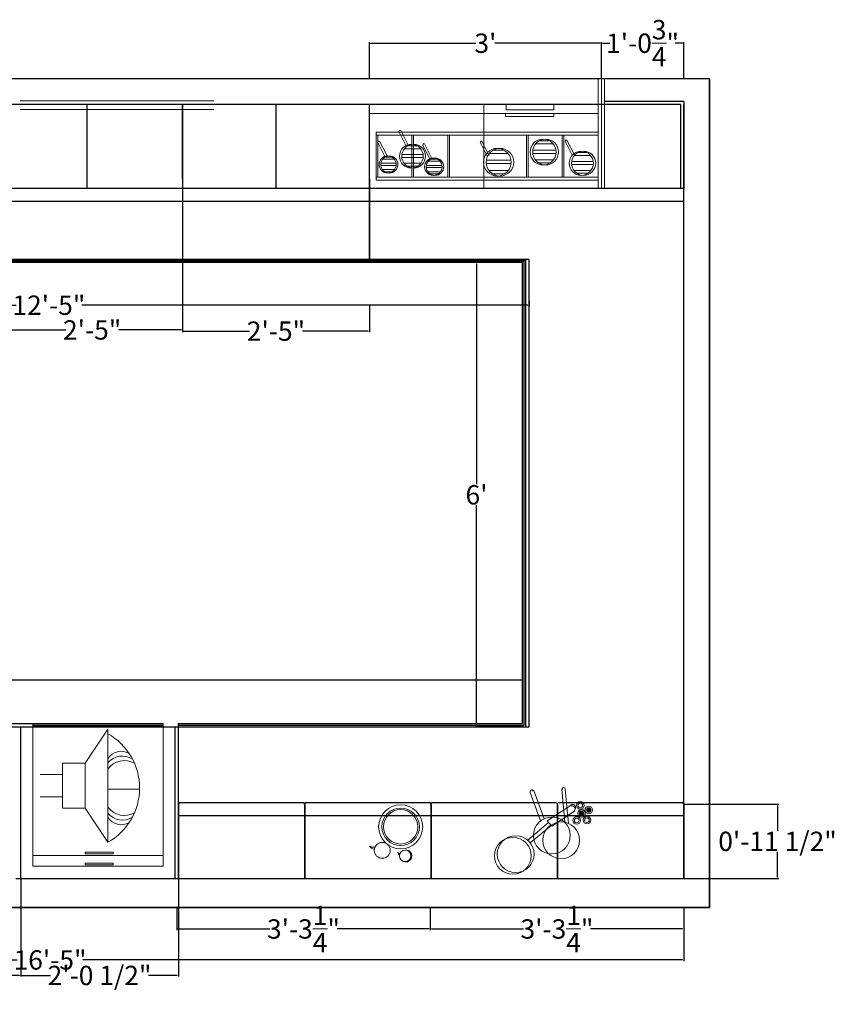
# Model space of a CAD drawing. Units: inches. Extents: x 1686244 to 1686928, y 1936095 to 1936489.
# Tile 11 of 11: x 1686801 to 1686928, y 1936330 to 1936483. Entities that reach past the tile are written whole.
import ezdxf

# ---------------------------------------------------------------- set-up
doc = ezdxf.new("R2010")
doc.units = ezdxf.units.IN
doc.header["$MEASUREMENT"] = 0
for name, color, linetype, lineweight in [('A-ANNO-DIMS', 240, 'Continuous', 18), ('A-CASE', 7, 'Continuous', 35), ('A-ELEV', 7, 'Continuous', 25), ('A-ELEV-PATT', 72, 'Continuous', 13), ('A-FURN', 40, 'Continuous', 18)]:
    doc.layers.add(name, color=color, linetype=linetype, lineweight=lineweight)
doc.styles.get("Standard").update_dxf_attribs({"font": 'arial.ttf'})
doc.dimstyles.get("Standard").update_dxf_attribs({"dimtxt": 3, "dimasz": 0.18, "dimexe": 0.18, "dimexo": 0.0625, "dimgap": 0.09, "dimtad": 0, "dimtih": 1, "dimtoh": 1, "dimzin": 0, "dimdsep": 46, "dimlunit": 4, "dimtxsty": 'Standard', "dimcen": 0.09, "dimadec": 0, "dimazin": 0, "dimtfac": 1, "dimtofl": 0, "dimtmove": 0, "dimatfit": 3, "dimfxl": 1, "dimtolj": 1, "dimtzin": 0, "dimarcsym": 0})

# ---------------------------------------------------------------- blocks, each defined once
blk = doc.blocks.new('*D21')
at = {"layer": 'A-ANNO-DIMS', "color": 0, "lineweight": -2, "transparency": 16777216}
for p, q in [((1686707.33, 1936344.88), (1686707.33, 1936336.62)), ((1686904.33, 1936344.88), (1686904.33, 1936336.62)), ((1686707.51, 1936336.8), (1686800.91, 1936336.8)), ((1686904.15, 1936336.8), (1686811.11, 1936336.8))]:
    blk.add_line(p, q, dxfattribs=at)
at = {"layer": 'A-ANNO-DIMS', "color": 0, "transparency": 16777216}
for points in [[(1686707.51, 1936336.83), (1686707.51, 1936336.77), (1686707.33, 1936336.8)], [(1686904.15, 1936336.83), (1686904.15, 1936336.77), (1686904.33, 1936336.8)]]:
    blk.add_solid(points, dxfattribs=at)
at = {"layer": 'Defpoints', "color": 0, "transparency": 16777216}
for p in [(1686707.33, 1936344.94), (1686904.33, 1936344.94), (1686904.33, 1936336.8)]:
    blk.add_point(p, dxfattribs=at)
at = {"layer": 'A-ANNO-DIMS', "color": 0, "transparency": 16777216, "insert": (1686806.01, 1936336.8), "char_height": 3, "attachment_point": 5}
blk.add_mtext('\\A1;16\'-5"', dxfattribs=at)
blk = doc.blocks.new('*D22')
at = {"layer": 'A-ANNO-DIMS', "color": 0, "lineweight": -2, "transparency": 16777216}
for p, q in [((1686865, 1936344.88), (1686865, 1936341.42)), ((1686904.33, 1936344.88), (1686904.33, 1936341.42)), ((1686865.18, 1936341.6), (1686879.45, 1936341.6)), ((1686904.15, 1936341.6), (1686889.88, 1936341.6))]:
    blk.add_line(p, q, dxfattribs=at)
at = {"layer": 'A-ANNO-DIMS', "color": 0, "transparency": 16777216}
for points in [[(1686865.18, 1936341.63), (1686865.18, 1936341.57), (1686865, 1936341.6)], [(1686904.15, 1936341.63), (1686904.15, 1936341.57), (1686904.33, 1936341.6)]]:
    blk.add_solid(points, dxfattribs=at)
at = {"layer": 'Defpoints', "color": 0, "transparency": 16777216}
for p in [(1686865, 1936344.94), (1686904.33, 1936344.94), (1686865, 1936341.6)]:
    blk.add_point(p, dxfattribs=at)
at = {"layer": 'A-ANNO-DIMS', "color": 0, "transparency": 16777216, "insert": (1686884.66, 1936341.6), "char_height": 3, "attachment_point": 5}
blk.add_mtext('\\A1;3\'-3{\\H1x;\\S1/4;}"', dxfattribs=at)
blk = doc.blocks.new('*D23')
at = {"layer": 'A-ANNO-DIMS', "color": 0, "lineweight": -2, "transparency": 16777216}
for p, q in [((1686825.67, 1936344.88), (1686825.67, 1936341.42)), ((1686865, 1936344.88), (1686865, 1936341.42)), ((1686825.85, 1936341.6), (1686840.12, 1936341.6)), ((1686864.82, 1936341.6), (1686850.55, 1936341.6))]:
    blk.add_line(p, q, dxfattribs=at)
at = {"layer": 'A-ANNO-DIMS', "color": 0, "transparency": 16777216}
for points in [[(1686825.85, 1936341.63), (1686825.85, 1936341.57), (1686825.67, 1936341.6)], [(1686864.82, 1936341.63), (1686864.82, 1936341.57), (1686865, 1936341.6)]]:
    blk.add_solid(points, dxfattribs=at)
at = {"layer": 'Defpoints', "color": 0, "transparency": 16777216}
for p in [(1686825.67, 1936344.94), (1686865, 1936344.94), (1686825.67, 1936341.6)]:
    blk.add_point(p, dxfattribs=at)
at = {"layer": 'A-ANNO-DIMS', "color": 0, "transparency": 16777216, "insert": (1686845.33, 1936341.6), "char_height": 3, "attachment_point": 5}
blk.add_mtext('\\A1;3\'-3{\\H1x;\\S1/4;}"', dxfattribs=at)
blk = doc.blocks.new('*D25')
at = {"layer": 'A-ANNO-DIMS', "color": 0, "lineweight": -2, "transparency": 16777216}
for p, q in [((1686879.26, 1936444.94), (1686872, 1936444.94)), ((1686872.18, 1936444.76), (1686872.18, 1936410.56)), ((1686872.18, 1936373.12), (1686872.18, 1936407.32)), ((1686879.4, 1936372.94), (1686872, 1936372.94))]:
    blk.add_line(p, q, dxfattribs=at)
at = {"layer": 'A-ANNO-DIMS', "color": 0, "transparency": 16777216}
for points in [[(1686872.15, 1936444.76), (1686872.21, 1936444.76), (1686872.18, 1936444.94)], [(1686872.15, 1936373.12), (1686872.21, 1936373.12), (1686872.18, 1936372.94)]]:
    blk.add_solid(points, dxfattribs=at)
at = {"layer": 'Defpoints', "color": 0, "transparency": 16777216}
for p in [(1686872.18, 1936444.94), (1686879.33, 1936444.94), (1686879.46, 1936372.94)]:
    blk.add_point(p, dxfattribs=at)
at = {"layer": 'A-ANNO-DIMS', "color": 0, "transparency": 16777216, "insert": (1686872.18, 1936408.94), "char_height": 3, "attachment_point": 5}
blk.add_mtext("\\A1;6'", dxfattribs=at)
blk = doc.blocks.new('*D26')
at = {"layer": 'A-ANNO-DIMS', "color": 0, "lineweight": -2, "transparency": 16777216}
for p, q in [((1686731.33, 1936439.01), (1686731.33, 1936438.16)), ((1686731.51, 1936438.34), (1686800.73, 1936438.34)), ((1686880.15, 1936438.34), (1686810.93, 1936438.34)), ((1686880.33, 1936439.01), (1686880.33, 1936438.16))]:
    blk.add_line(p, q, dxfattribs=at)
at = {"layer": 'A-ANNO-DIMS', "color": 0, "transparency": 16777216}
for points in [[(1686731.51, 1936438.37), (1686731.51, 1936438.31), (1686731.33, 1936438.34)], [(1686880.15, 1936438.37), (1686880.15, 1936438.31), (1686880.33, 1936438.34)]]:
    blk.add_solid(points, dxfattribs=at)
at = {"layer": 'Defpoints', "color": 0, "transparency": 16777216}
for p in [(1686731.33, 1936439.07), (1686731.33, 1936438.34), (1686880.33, 1936439.07)]:
    blk.add_point(p, dxfattribs=at)
at = {"layer": 'A-ANNO-DIMS', "color": 0, "transparency": 16777216, "insert": (1686805.83, 1936438.34), "char_height": 3, "attachment_point": 5}
blk.add_mtext('\\A1;12\'-5"', dxfattribs=at)
blk = doc.blocks.new('*D29')
at = {"layer": 'A-ANNO-DIMS', "color": 0, "lineweight": -2, "transparency": 16777216}
for p, q in [((1686797.56, 1936438.28), (1686797.56, 1936434.32)), ((1686826.56, 1936438.28), (1686826.56, 1936434.32)), ((1686797.74, 1936434.5), (1686808.44, 1936434.5)), ((1686826.38, 1936434.5), (1686816.65, 1936434.5))]:
    blk.add_line(p, q, dxfattribs=at)
at = {"layer": 'A-ANNO-DIMS', "color": 0, "transparency": 16777216}
for points in [[(1686797.74, 1936434.53), (1686797.74, 1936434.47), (1686797.56, 1936434.5)], [(1686826.38, 1936434.53), (1686826.38, 1936434.47), (1686826.56, 1936434.5)]]:
    blk.add_solid(points, dxfattribs=at)
at = {"layer": 'Defpoints', "color": 0, "transparency": 16777216}
for p in [(1686797.56, 1936438.34), (1686826.56, 1936438.34), (1686826.56, 1936434.5)]:
    blk.add_point(p, dxfattribs=at)
at = {"layer": 'A-ANNO-DIMS', "color": 0, "transparency": 16777216, "insert": (1686812.54, 1936434.5), "char_height": 3, "attachment_point": 5}
blk.add_mtext('\\A1;2\'-5"', dxfattribs=at)
blk = doc.blocks.new('*D30')
at = {"layer": 'A-ANNO-DIMS', "color": 0, "lineweight": -2, "transparency": 16777216}
for p, q in [((1686826.56, 1936438.28), (1686826.56, 1936434.14)), ((1686855.56, 1936438.28), (1686855.56, 1936434.14)), ((1686826.74, 1936434.32), (1686836.95, 1936434.32)), ((1686855.38, 1936434.32), (1686845.16, 1936434.32))]:
    blk.add_line(p, q, dxfattribs=at)
at = {"layer": 'A-ANNO-DIMS', "color": 0, "transparency": 16777216}
for points in [[(1686826.74, 1936434.35), (1686826.74, 1936434.29), (1686826.56, 1936434.32)], [(1686855.38, 1936434.35), (1686855.38, 1936434.29), (1686855.56, 1936434.32)]]:
    blk.add_solid(points, dxfattribs=at)
at = {"layer": 'Defpoints', "color": 0, "transparency": 16777216}
for p in [(1686826.56, 1936438.34), (1686855.56, 1936438.34), (1686855.56, 1936434.32)]:
    blk.add_point(p, dxfattribs=at)
at = {"layer": 'A-ANNO-DIMS', "color": 0, "transparency": 16777216, "insert": (1686841.06, 1936434.32), "char_height": 3, "attachment_point": 5}
blk.add_mtext('\\A1;2\'-5"', dxfattribs=at)
blk = doc.blocks.new('*D31')
at = {"layer": 'A-ANNO-DIMS', "color": 0, "lineweight": -2, "transparency": 16777216}
for p, q in [((1686855.56, 1936473.5), (1686855.56, 1936479.15)), ((1686891.56, 1936473.5), (1686891.56, 1936479.15)), ((1686855.74, 1936478.97), (1686872.09, 1936478.97)), ((1686891.38, 1936478.97), (1686875.03, 1936478.97))]:
    blk.add_line(p, q, dxfattribs=at)
at = {"layer": 'A-ANNO-DIMS', "color": 0, "transparency": 16777216}
for points in [[(1686855.74, 1936479), (1686855.74, 1936478.94), (1686855.56, 1936478.97)], [(1686891.38, 1936479), (1686891.38, 1936478.94), (1686891.56, 1936478.97)]]:
    blk.add_solid(points, dxfattribs=at)
at = {"layer": 'Defpoints', "color": 0, "transparency": 16777216}
for p in [(1686891.56, 1936478.97), (1686855.56, 1936473.44), (1686891.56, 1936473.44)]:
    blk.add_point(p, dxfattribs=at)
at = {"layer": 'A-ANNO-DIMS', "color": 0, "transparency": 16777216, "insert": (1686873.56, 1936478.97), "char_height": 3, "attachment_point": 5}
blk.add_mtext("\\A1;3'", dxfattribs=at)
blk = doc.blocks.new('*D32')
at = {"layer": 'A-ANNO-DIMS', "color": 0, "lineweight": -2, "transparency": 16777216}
for p, q in [((1686891.56, 1936473.5), (1686891.56, 1936479.15)), ((1686904.33, 1936473.5), (1686904.33, 1936479.15)), ((1686891.74, 1936478.97), (1686892.87, 1936478.97)), ((1686904.15, 1936478.97), (1686903.02, 1936478.97))]:
    blk.add_line(p, q, dxfattribs=at)
at = {"layer": 'A-ANNO-DIMS', "color": 0, "transparency": 16777216}
for points in [[(1686891.74, 1936479), (1686891.74, 1936478.94), (1686891.56, 1936478.97)], [(1686904.15, 1936479), (1686904.15, 1936478.94), (1686904.33, 1936478.97)]]:
    blk.add_solid(points, dxfattribs=at)
at = {"layer": 'Defpoints', "color": 0, "transparency": 16777216}
for p in [(1686904.33, 1936478.97), (1686891.56, 1936473.44), (1686904.33, 1936473.44)]:
    blk.add_point(p, dxfattribs=at)
at = {"layer": 'A-ANNO-DIMS', "color": 0, "transparency": 16777216, "insert": (1686897.94, 1936478.97), "char_height": 3, "attachment_point": 5}
blk.add_mtext('\\A1;1\'-0{\\H1x;\\S3/4;}"', dxfattribs=at)
blk = doc.blocks.new('*D35')
at = {"layer": 'A-ANNO-DIMS', "color": 0, "lineweight": -2, "transparency": 16777216}
for p, q in [((1686707.33, 1936377.76), (1686707.33, 1936380.38)), ((1686707.51, 1936380.2), (1686788.23, 1936380.2)), ((1686879.15, 1936380.2), (1686798.43, 1936380.2)), ((1686879.33, 1936377.76), (1686879.33, 1936380.38))]:
    blk.add_line(p, q, dxfattribs=at)
at = {"layer": 'A-ANNO-DIMS', "color": 0, "transparency": 16777216}
for points in [[(1686707.51, 1936380.23), (1686707.51, 1936380.17), (1686707.33, 1936380.2)], [(1686879.15, 1936380.23), (1686879.15, 1936380.17), (1686879.33, 1936380.2)]]:
    blk.add_solid(points, dxfattribs=at)
at = {"layer": 'Defpoints', "color": 0, "transparency": 16777216}
for p in [(1686879.33, 1936380.2), (1686707.33, 1936377.7), (1686879.33, 1936377.7)]:
    blk.add_point(p, dxfattribs=at)
at = {"layer": 'A-ANNO-DIMS', "color": 0, "transparency": 16777216, "insert": (1686793.33, 1936380.2), "char_height": 3, "attachment_point": 5}
blk.add_mtext('\\A1;14\'-4"', dxfattribs=at)
blk = doc.blocks.new('*D108')
at = {"layer": 'A-ANNO-DIMS', "color": 0, "lineweight": -2, "transparency": 16777216}
for p, q in [((1686776.77, 1936349.38), (1686776.77, 1936334.21)), ((1686801.47, 1936349.38), (1686801.47, 1936334.21)), ((1686776.95, 1936334.39), (1686781.52, 1936334.39)), ((1686801.29, 1936334.39), (1686796.72, 1936334.39))]:
    blk.add_line(p, q, dxfattribs=at)
at = {"layer": 'A-ANNO-DIMS', "color": 0, "transparency": 16777216}
for points in [[(1686776.95, 1936334.42), (1686776.95, 1936334.36), (1686776.77, 1936334.39)], [(1686801.29, 1936334.42), (1686801.29, 1936334.36), (1686801.47, 1936334.39)]]:
    blk.add_solid(points, dxfattribs=at)
at = {"layer": 'Defpoints', "color": 0, "transparency": 16777216}
for p in [(1686776.77, 1936349.44), (1686801.47, 1936349.44), (1686801.47, 1936334.39)]:
    blk.add_point(p, dxfattribs=at)
at = {"layer": 'A-ANNO-DIMS', "color": 0, "transparency": 16777216, "insert": (1686789.12, 1936334.39), "char_height": 3, "attachment_point": 5}
blk.add_mtext('\\A1;2\'-0 1/2"', dxfattribs=at)
blk = doc.blocks.new('*D109')
at = {"layer": 'A-ANNO-DIMS', "color": 0, "lineweight": -2, "transparency": 16777216}
for p, q in [((1686801.47, 1936349.38), (1686801.47, 1936334.21)), ((1686825.92, 1936349.38), (1686825.92, 1936334.21)), ((1686801.65, 1936334.39), (1686806.1, 1936334.39)), ((1686825.74, 1936334.39), (1686821.29, 1936334.39))]:
    blk.add_line(p, q, dxfattribs=at)
at = {"layer": 'A-ANNO-DIMS', "color": 0, "transparency": 16777216}
for points in [[(1686801.65, 1936334.42), (1686801.65, 1936334.36), (1686801.47, 1936334.39)], [(1686825.74, 1936334.42), (1686825.74, 1936334.36), (1686825.92, 1936334.39)]]:
    blk.add_solid(points, dxfattribs=at)
at = {"layer": 'Defpoints', "color": 0, "transparency": 16777216}
for p in [(1686801.47, 1936349.44), (1686825.92, 1936349.44), (1686825.92, 1936334.39)]:
    blk.add_point(p, dxfattribs=at)
at = {"layer": 'A-ANNO-DIMS', "color": 0, "transparency": 16777216, "insert": (1686813.69, 1936334.39), "char_height": 3, "attachment_point": 5}
blk.add_mtext('\\A1;2\'-0 1/2"', dxfattribs=at)
blk = doc.blocks.new('*D112')
at = {"layer": 'A-ANNO-DIMS', "color": 0, "lineweight": -2, "transparency": 16777216}
for p, q in [((1686904.39, 1936360.94), (1686919.06, 1936360.94)), ((1686918.88, 1936360.76), (1686918.88, 1936356.83)), ((1686918.88, 1936349.62), (1686918.88, 1936353.55)), ((1686904.39, 1936349.44), (1686919.06, 1936349.44))]:
    blk.add_line(p, q, dxfattribs=at)
at = {"layer": 'A-ANNO-DIMS', "color": 0, "transparency": 16777216}
for points in [[(1686918.85, 1936360.76), (1686918.91, 1936360.76), (1686918.88, 1936360.94)], [(1686918.85, 1936349.62), (1686918.91, 1936349.62), (1686918.88, 1936349.44)]]:
    blk.add_solid(points, dxfattribs=at)
at = {"layer": 'Defpoints', "color": 0, "transparency": 16777216}
for p in [(1686904.33, 1936360.94), (1686904.33, 1936349.44), (1686918.88, 1936349.44)]:
    blk.add_point(p, dxfattribs=at)
at = {"layer": 'A-ANNO-DIMS', "color": 0, "transparency": 16777216, "insert": (1686918.88, 1936355.19), "char_height": 3, "attachment_point": 5}
blk.add_mtext('\\A1;0\'-11 1/2"', dxfattribs=at)

msp = doc.modelspace()

# ---------------------------------------------------------------- hatches: boundary and pattern name
at = {"layer": 'A-ELEV-PATT'}
h = msp.add_hatch(dxfattribs=at)
h.set_pattern_fill('ANSI32', color=256, scale=3.918348, angle=135)
h.set_pattern_definition([(180, (-855412.5119, -981919.0557), (-2e-16, -1.46938062567), []), (180, (-855413.0017, -981918.5659), (-2e-16, -1.46938062567), [])])
h.paths.add_polyline_path([(1686882.705, 1936460.094, 0.3861806), (1686884.519, 1936462.092, 0.3861806), (1686882.705, 1936464.09, 0.3861806), (1686880.892, 1936462.092, 0.3861806)])
h = msp.add_hatch(dxfattribs=at)
h.set_pattern_fill('ANSI32', color=256, scale=3.601818, angle=135)
h.set_pattern_definition([(180, (-650062.0521, -746167.9158), (-2e-16, -1.3506815667), []), (180, (-650062.5023, -746167.4655), (-2e-16, -1.3506815667), [])])
h.paths.add_polyline_path([(1686862.246, 1936459.617, 0.3861806), (1686863.913, 1936461.453, 0.3861806), (1686862.246, 1936463.29, 0.3861806), (1686860.579, 1936461.453, 0.3861806)])
h = msp.add_hatch(dxfattribs=at)
h.set_pattern_fill('ANSI32', color=256, scale=4.184979, angle=135)
h.set_pattern_definition([(180, (-1028414.4015, -1180506.824), (-2e-16, -1.5693671227), []), (180, (-1028414.9246, -1180506.3008), (-2e-16, -1.5693671227), [])])
h.paths.add_polyline_path([(1686875.606, 1936458.385, 0.3861806), (1686877.543, 1936460.519, 0.3861806), (1686875.606, 1936462.653, 0.3861806), (1686873.669, 1936460.519, 0.3861806)])
h = msp.add_hatch(dxfattribs=at)
h.set_pattern_fill('ANSI32', color=256, scale=2.6, angle=135)
h.set_pattern_definition([(180, (-68.4762, -16.7264), (-1e-16, -0.975), []), (180, (-68.8012, -16.4014), (-1e-16, -0.975), [])])
h.paths.add_polyline_path([(1686858.514, 1936458.834, 0.3861806), (1686859.718, 1936460.16, 0.3861806), (1686858.514, 1936461.486, 0.3861806), (1686857.311, 1936460.16, 0.3861806)])
h = msp.add_hatch(dxfattribs=at)
h.set_pattern_fill('ANSI32', color=256, scale=2.637795, angle=135)
h.set_pattern_definition([(180, (-24583.2303, -28166.474), (-1e-16, -0.98917299), []), (180, (-24583.5601, -28166.1443), (-1e-16, -0.98917299), [])])
h.paths.add_polyline_path([(1686865.606, 1936458.47, 0.3861806), (1686866.827, 1936459.815, 0.3861806), (1686865.606, 1936461.16, 0.3861806), (1686864.385, 1936459.815, 0.3861806)])
h = msp.add_hatch(dxfattribs=at)
h.set_pattern_fill('ANSI32', color=256, scale=3.669954, angle=135)
h.set_pattern_definition([(180, (-694244.093, -796917.2364), (-2e-16, -1.3762328775), []), (180, (-694244.5517, -796916.7777), (-2e-16, -1.3762328775), [])])
h.paths.add_polyline_path([(1686888.611, 1936458.49, 0.3861806), (1686890.31, 1936460.361, 0.3861806), (1686888.611, 1936462.232, 0.3861806), (1686886.912, 1936460.361, 0.3861806)])

# ---------------------------------------------------------------- linework, layer by layer
at = {"layer": 'A-CASE'}
for p, q in [((1686908.327, 1936344.942), (1686908.327, 1936473.442)), ((1686703.327, 1936344.942), (1686908.327, 1936344.942))]:
    msp.add_line(p, q, dxfattribs=at)
at = {"layer": 'A-ELEV'}
for p, q in [((1686908.327, 1936473.442), (1686703.327, 1936473.442)), ((1686903.827, 1936469.442), (1686707.327, 1936469.442)), ((1686811.775, 1936456.442), (1686811.775, 1936469.442)), ((1686826.556, 1936457.879), (1686826.556, 1936469.442)), ((1686826.556, 1936469.442), (1686826.556, 1936438.341)), ((1686841.106, 1936456.442), (1686841.106, 1936469.442)), ((1686855.556, 1936444.942), (1686855.556, 1936469.442)), ((1686904.327, 1936469.942), (1686892.056, 1936469.942)), ((1686903.827, 1936469.442), (1686903.827, 1936456.442)), ((1686904.327, 1936469.942), (1686904.327, 1936456.442)), ((1686904.327, 1936349.442), (1686904.327, 1936469.442)), ((1686855.556, 1936457.909), (1686855.556, 1936444.942)), ((1686904.327, 1936456.442), (1686731.327, 1936456.442)), ((1686904.327, 1936454.442), (1686731.327, 1936454.442)), ((1686880.327, 1936445.442), (1686731.327, 1936445.442)), ((1686879.827, 1936445.342), (1686731.327, 1936445.342)), ((1686879.577, 1936445.097), (1686731.327, 1936445.097)), ((1686879.327, 1936444.942), (1686731.327, 1936444.942)), ((1686879.327, 1936373.442), (1686879.327, 1936444.942)), ((1686879.577, 1936373.192), (1686879.577, 1936445.342)), ((1686879.827, 1936372.942), (1686879.827, 1936445.342)), ((1686880.327, 1936372.942), (1686880.327, 1936445.442)), ((1686752.327, 1936373.442), (1686823.58, 1936373.442)), ((1686752.327, 1936372.942), (1686880.327, 1936372.942)), ((1686801.471, 1936349.442), (1686801.471, 1936372.942)), ((1686825.419, 1936349.442), (1686825.419, 1936372.942)), ((1686825.919, 1936349.442), (1686825.919, 1936373.442)), ((1686825.919, 1936373.442), (1686879.327, 1936373.442)), ((1686825.919, 1936373.192), (1686879.577, 1936373.192)), ((1686826.169, 1936361.192), (1686845.271, 1936361.192)), ((1686845.771, 1936361.192), (1686864.873, 1936361.192)), ((1686865.373, 1936361.192), (1686884.475, 1936361.192)), ((1686884.975, 1936361.192), (1686904.077, 1936361.192)), ((1686904.327, 1936360.942), (1686904.327, 1936349.442)), ((1686825.919, 1936359.192), (1686904.327, 1936359.192)), ((1686800.704, 1936349.442), (1686904.327, 1936349.442))]:
    msp.add_line(p, q, dxfattribs=at)
at = {"layer": 'A-ELEV', "const_width": 0.25}
for points in [[(1686825.919, 1936360.942), (1686825.919, 1936349.442)], [(1686845.521, 1936360.942), (1686845.521, 1936349.442)], [(1686865.123, 1936360.942), (1686865.123, 1936349.442)], [(1686884.725, 1936360.942), (1686884.725, 1936349.442)]]:
    msp.add_lwpolyline(points, dxfattribs=at)
at = {"layer": 'A-ELEV'}
for centre, start, end in [((1686826.169, 1936360.942), 90, 180), ((1686845.271, 1936360.942), 0, 90), ((1686845.771, 1936360.942), 90, 180), ((1686864.873, 1936360.942), 0, 90), ((1686865.373, 1936360.942), 90, 180), ((1686904.077, 1936360.942), 0, 90)]:
    msp.add_arc(centre, 0.25, start, end, dxfattribs=at)
at = {"layer": 'A-FURN'}
for p, q in [((1686891.056, 1936473.442), (1686891.056, 1936456.442)), ((1686891.556, 1936473.442), (1686891.556, 1936456.442)), ((1686892.056, 1936473.442), (1686892.056, 1936456.442)), ((1686801.392, 1936470.034), (1686831.445, 1936470.034)), ((1686801.392, 1936468.712), (1686831.445, 1936468.712)), ((1686873.306, 1936456.442), (1686873.306, 1936469.442)), ((1686855.556, 1936468.059), (1686891.056, 1936468.059)), ((1686861.564, 1936463.164), (1686860.415, 1936465.436)), ((1686857.097, 1936464.701), (1686856.597, 1936464.701)), ((1686856.597, 1936464.701), (1686873.306, 1936464.701)), ((1686856.847, 1936464.701), (1686856.847, 1936458.206)), ((1686861.227, 1936463.096), (1686860.183, 1936465.159)), ((1686862.167, 1936464.701), (1686862.167, 1936458.206)), ((1686862.417, 1936464.701), (1686862.417, 1936458.206)), ((1686867.736, 1936464.701), (1686867.736, 1936458.206)), ((1686867.986, 1936464.701), (1686867.986, 1936458.206)), ((1686879.917, 1936464.701), (1686879.917, 1936458.206)), ((1686880.167, 1936464.701), (1686880.167, 1936458.206)), ((1686885.486, 1936464.701), (1686885.486, 1936458.206)), ((1686885.736, 1936464.701), (1686885.736, 1936458.206)), ((1686887.365, 1936461.682), (1686886.216, 1936463.953)), ((1686857.955, 1936461.42), (1686856.912, 1936463.484)), ((1686858.293, 1936461.489), (1686857.144, 1936463.76)), ((1686864.914, 1936461.044), (1686863.871, 1936463.108)), ((1686865.252, 1936461.112), (1686864.103, 1936463.384)), ((1686873.827, 1936461.453), (1686872.783, 1936463.517)), ((1686874.164, 1936461.521), (1686873.015, 1936463.793)), ((1686887.027, 1936461.613), (1686885.984, 1936463.677)), ((1686857.097, 1936458.206), (1686856.597, 1936458.206)), ((1686811.474, 1936367.336), (1686814.986, 1936372.603)), ((1686814.986, 1936355.046), (1686814.986, 1936372.603)), ((1686811.474, 1936367.336), (1686807.963, 1936367.336)), ((1686807.963, 1936367.336), (1686807.963, 1936360.313)), ((1686811.474, 1936360.313), (1686811.474, 1936367.336)), ((1686807.963, 1936365.58), (1686804.452, 1936365.58)), ((1686814.986, 1936363.289), (1686819.897, 1936363.289)), ((1686882.659, 1936358.693), (1686881.051, 1936363.082)), ((1686885.86, 1936358.156), (1686885.43, 1936363.303)), ((1686885.947, 1936363.303), (1686886.446, 1936357.975)), ((1686804.452, 1936362.069), (1686807.963, 1936362.069)), ((1686882.115, 1936358.36), (1686880.506, 1936362.748)), ((1686807.963, 1936360.313), (1686811.474, 1936360.313)), ((1686814.986, 1936355.046), (1686811.474, 1936360.313)), ((1686883.142, 1936358.367), (1686886.712, 1936360.68)), ((1686889.513, 1936360.072), (1686889.251, 1936360.128)), ((1686889.513, 1936360.035), (1686889.251, 1936359.979)), ((1686889.528, 1936360.107), (1686889.312, 1936360.264)), ((1686889.556, 1936360.132), (1686889.422, 1936360.364)), ((1686889.592, 1936360.144), (1686889.564, 1936360.41)), ((1686889.63, 1936360.14), (1686889.712, 1936360.394)), ((1686889.662, 1936360.121), (1686889.841, 1936360.32)), ((1686889.685, 1936360.09), (1686889.929, 1936360.199)), ((1686889.685, 1936360.017), (1686889.929, 1936359.908)), ((1686889.692, 1936360.054), (1686889.96, 1936360.054)), ((1686883.841, 1936357.559), (1686887.386, 1936359.891)), ((1686888.384, 1936359.548), (1686888.123, 1936359.604)), ((1686888.384, 1936359.51), (1686888.123, 1936359.455)), ((1686888.4, 1936359.583), (1686888.183, 1936359.74)), ((1686888.4, 1936359.476), (1686888.183, 1936359.319)), ((1686888.428, 1936359.608), (1686888.294, 1936359.84)), ((1686888.428, 1936359.451), (1686888.294, 1936359.219)), ((1686888.464, 1936359.62), (1686888.436, 1936359.886)), ((1686888.464, 1936359.439), (1686888.436, 1936359.173)), ((1686888.501, 1936359.616), (1686888.584, 1936359.87)), ((1686888.501, 1936359.443), (1686888.584, 1936359.189)), ((1686888.534, 1936359.597), (1686888.713, 1936359.796)), ((1686888.534, 1936359.462), (1686888.713, 1936359.263)), ((1686888.556, 1936359.566), (1686888.8, 1936359.675)), ((1686888.556, 1936359.492), (1686888.8, 1936359.384)), ((1686888.564, 1936359.529), (1686888.831, 1936359.529)), ((1686889.528, 1936360), (1686889.312, 1936359.843)), ((1686889.556, 1936359.975), (1686889.422, 1936359.743)), ((1686889.592, 1936359.963), (1686889.564, 1936359.697)), ((1686889.63, 1936359.967), (1686889.712, 1936359.713)), ((1686889.662, 1936359.986), (1686889.841, 1936359.787)), ((1686880.122, 1936355.373), (1686883.357, 1936358.113)), ((1686880.507, 1936354.968), (1686883.756, 1936357.656)), ((1686883.357, 1936358.113), (1686883.142, 1936358.367)), ((1686883.841, 1936357.559), (1686883.357, 1936358.113)), ((1686803.322, 1936353.022), (1686823.58, 1936353.022))]:
    msp.add_line(p, q, dxfattribs=at)
for points in [[(1686876.785, 1936469.442), (1686884.183, 1936469.442), (1686884.183, 1936468.656), (1686876.785, 1936468.656)], [(1686876.694, 1936468.059), (1686884.183, 1936468.059), (1686884.183, 1936467.63), (1686876.694, 1936467.63)], [(1686856.597, 1936465.201), (1686891.056, 1936465.201), (1686891.056, 1936457.706), (1686856.597, 1936457.706)], [(1686803.322, 1936373.442), (1686823.58, 1936373.442), (1686823.58, 1936351.331), (1686803.322, 1936351.331)], [(1686811.453, 1936353.524), (1686815.803, 1936353.524), (1686815.803, 1936353.234), (1686811.453, 1936353.234)], [(1686811.453, 1936351.82), (1686815.803, 1936351.82), (1686815.803, 1936351.531), (1686811.453, 1936351.531)]]:
    msp.add_lwpolyline(points, close=True, dxfattribs=at)
for points in [[(1686857.097, 1936464.701), (1686891.056, 1936464.701)], [(1686891.056, 1936458.206), (1686857.097, 1936458.206)]]:
    msp.add_lwpolyline(points, dxfattribs=at)
at = {"layer": 'A-FURN', "const_width": 0.25}
msp.add_lwpolyline([(1686803.322, 1936373.179), (1686823.58, 1936373.179)], dxfattribs=at)
at = {"layer": 'A-FURN'}
for centre, radius in [((1686882.512, 1936462.092), 2.007), ((1686882.899, 1936462.092), 2.007), ((1686862.068, 1936461.453), 1.845), ((1686862.424, 1936461.453), 1.845), ((1686875.399, 1936460.519), 2.144), ((1686875.813, 1936460.519), 2.144), ((1686858.386, 1936460.16), 1.332), ((1686858.643, 1936460.16), 1.332), ((1686865.475, 1936459.815), 1.351), ((1686865.736, 1936459.815), 1.351), ((1686888.43, 1936460.361), 1.88), ((1686888.792, 1936460.361), 1.88), ((1686880.881, 1936363.063), 0.058), ((1686885.473, 1936363.33), 0.0404), ((1686860.41, 1936357.443), 3.415), ((1686860.41, 1936357.443), 2.915), ((1686860.41, 1936357.443), 2.665), ((1686888.288, 1936360.768), 0.587), ((1686888.473, 1936359.529), 0.587), ((1686888.288, 1936360.768), 0.358), ((1686889.602, 1936360.054), 0.587), ((1686889.602, 1936360.054), 0.358), ((1686889.602, 1936360.054), 0.0908), ((1686883.87, 1936356.104), 2.858), ((1686887.732, 1936358.437), 0.587), ((1686887.732, 1936358.437), 0.358), ((1686888.473, 1936359.529), 0.358), ((1686888.473, 1936359.529), 0.0908), ((1686889.315, 1936358.485), 0.587), ((1686889.315, 1936358.485), 0.358), ((1686885.317, 1936355.35), 2.858), ((1686877.821, 1936352.955), 2.858), ((1686878.253, 1936353.212), 2.858), ((1686857.552, 1936353.787), 1.23), ((1686861.118, 1936352.952), 0.893)]:
    msp.add_circle(centre, radius, dxfattribs=at)
for centre, radius, start, end in [((1686860.337, 1936465.265), 0.187, 65.40581, 214.5723), ((1686886.138, 1936463.783), 0.187, 65.40581, 214.5723), ((1686857.066, 1936463.59), 0.187, 65.40581, 214.5723), ((1686864.025, 1936463.214), 0.187, 65.40581, 214.5723), ((1686872.937, 1936463.623), 0.187, 65.40581, 214.5723), ((1686810.237, 1936363.46), 9.662, 299.43944, 60.56056), ((1686817.055, 1936366.727), 2.43, 60.09039, 148.36141), ((1686817.222, 1936365.502), 2.922, 57.7978, 139.95062), ((1686817.533, 1936364.596), 3.126, 59.86609, 144.59682), ((1686880.82, 1936362.848), 0.329, 45.31397, 197.64967), ((1686885.688, 1936363.303), 0.259, 0, 180), ((1686817.533, 1936362.324), 3.126, 215.40318, 300.13391), ((1686884.475, 1936360.942), 0.25, 0, 90), ((1686884.975, 1936360.942), 0.25, 90, 180), ((1686887.108, 1936360.456), 0.455, 320.72145, 150.51859), ((1686886.911, 1936360.168), 0.55, 329.69008, 111.24004), ((1686817.222, 1936361.418), 2.922, 220.04938, 302.2022), ((1686817.055, 1936360.194), 2.43, 211.63859, 299.90961), ((1686856.445, 1936355.023), 1.034, 213.44944, 264.20204), ((1686856.387, 1936356.1), 1.832, 243.95895, 271.05946), ((1686860.317, 1936353.469), 0.35, 178.70944, 257.58249), ((1686860.206, 1936353.553), 0.251, 197.81344, 293.15493), ((1686860.206, 1936353.553), 0.251, 0.0117442645317992, 0.0117443708500602), ((1686861.22, 1936352.919), 0.932, 228.35416, 96.31644)]:
    msp.add_arc(centre, radius, start, end, dxfattribs=at)
for p in [(1686862.167, 1936464.701), (1686867.736, 1936464.701)]:
    msp.add_point(p, dxfattribs=at)

# ---------------------------------------------------------------- dimensions: what is measured, and where the dimension line sits
at = {"layer": 'A-ANNO-DIMS'}
for base, p1, p2, override, picture, middle in [((1686904.327, 1936478.966), (1686891.556, 1936473.442), (1686904.327, 1936473.442), {"dimclrd": 0, "dimclre": 0, "dimclrt": 0}, '*D32', (1686897.942, 1936478.966)), ((1686891.556, 1936478.966), (1686855.556, 1936473.442), (1686891.556, 1936473.442), {"dimclrd": 0, "dimclre": 0, "dimclrt": 0}, '*D31', (1686873.556, 1936478.966)), ((1686731.327, 1936438.341), (1686880.327, 1936439.075), (1686731.327, 1936439.075), {"dimclrd": 0, "dimclre": 0, "dimclrt": 0}, '*D26', (1686805.827, 1936438.341)), ((1686801.471, 1936334.392), (1686776.774, 1936349.442), (1686801.471, 1936349.442), {"dimdec": 1, "dimlfac": 1, "dimrnd": 0, "dimzin": 1, "dimdsep": 46, "dimlunit": 4, "dimfrac": 2}, '*D108', (1686789.123, 1936334.392)), ((1686825.919, 1936334.392), (1686801.471, 1936349.442), (1686825.919, 1936349.442), {"dimdec": 1, "dimlfac": 1, "dimrnd": 0, "dimzin": 1, "dimdsep": 46, "dimlunit": 4, "dimfrac": 2}, '*D109', (1686813.695, 1936334.392)), ((1686825.669, 1936341.604), (1686864.998, 1936344.942), (1686825.669, 1936344.942), {"dimclrd": 0, "dimclre": 0, "dimclrt": 0}, '*D23', (1686845.333, 1936341.604)), ((1686864.998, 1936341.604), (1686904.327, 1936344.942), (1686864.998, 1936344.942), {"dimclrd": 0, "dimclre": 0, "dimclrt": 0}, '*D22', (1686884.663, 1936341.604))]:
    dim = msp.add_linear_dim(base=base, p1=p1, p2=p2, dimstyle='Standard', override=override, dxfattribs=at)
    dim.commit()
    dim.dimension.update_dxf_attribs({"geometry": picture, "text_midpoint": middle})
dim = msp.add_linear_dim(base=(1686872.18, 1936444.942), p1=(1686879.464, 1936372.942), p2=(1686879.327, 1936444.942), angle=90, dimstyle='Standard', override={"dimclrd": 0, "dimclre": 0, "dimclrt": 0}, dxfattribs=at)
dim.commit()
dim.dimension.update_dxf_attribs({"geometry": '*D25', "text_midpoint": (1686872.18, 1936408.942), "dimtype": 160})
for base, p1, p2, picture, middle in [((1686826.556, 1936434.502), (1686797.556, 1936438.341), (1686826.556, 1936438.341), '*D29', (1686812.543, 1936434.502)), ((1686855.556, 1936434.322), (1686826.556, 1936438.341), (1686855.556, 1936438.341), '*D30', (1686841.056, 1936434.322)), ((1686879.327, 1936380.203), (1686707.327, 1936377.699), (1686879.327, 1936377.699), '*D35', (1686793.327, 1936380.203)), ((1686904.327, 1936336.8), (1686707.327, 1936344.942), (1686904.327, 1936344.942), '*D21', (1686806.007, 1936336.8))]:
    dim = msp.add_linear_dim(base=base, p1=p1, p2=p2, dimstyle='Standard', override={"dimclrd": 0, "dimclre": 0, "dimclrt": 0}, dxfattribs=at)
    dim.commit()
    dim.dimension.update_dxf_attribs({"geometry": picture, "text_midpoint": middle, "dimtype": 160})
dim = msp.add_linear_dim(base=(1686918.877, 1936349.442), p1=(1686904.327, 1936360.942), p2=(1686904.327, 1936349.442), angle=90, dimstyle='Standard', override={"dimdec": 1, "dimlfac": 1, "dimrnd": 0, "dimzin": 1, "dimdsep": 46, "dimlunit": 4, "dimfrac": 2}, dxfattribs=at)
dim.commit()
dim.dimension.update_dxf_attribs({"geometry": '*D112', "text_midpoint": (1686918.877, 1936355.192)})

doc.saveas('drawing.dxf')
